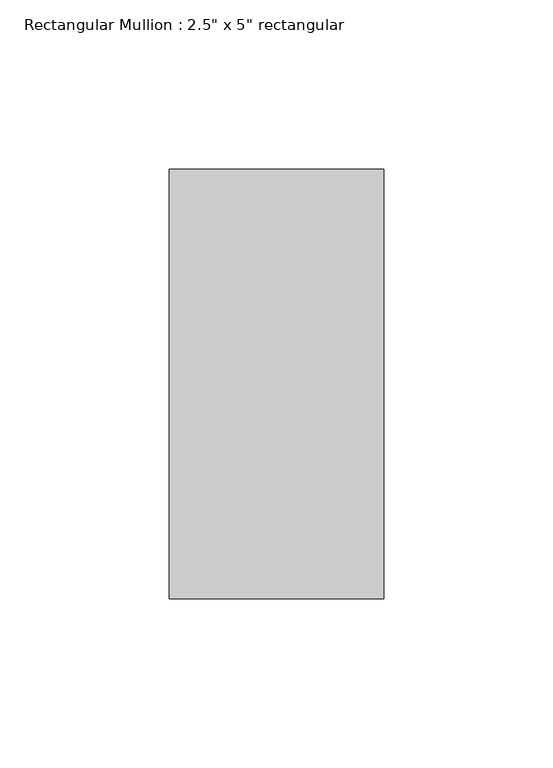
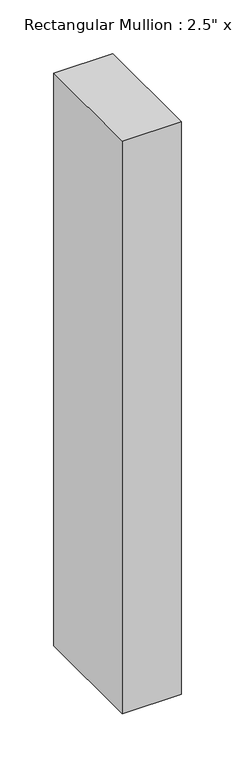
"""IFC4 building model written with IfcOpenShell, lengths in millimetres: member geometry."""

from ifc_helpers import new_model, si_unit, frame, origin, place, context, project, spatial, polyline, outline, extrude, source, transform, mapped, element, save


def member_1d9ef59f(model_context):
    return source(origin(), model_context, "Body", "SweptSolid", [
        extrude(outline(polyline([(0.0, 63.5), (0.0, -63.5), (-63.5, -63.5), (-63.5, 63.5), (0.0, 63.5)])), frame((0.0, 0.0, -650.4541417), z_axis=(0.0, 0.0, 1.0), x_axis=(1.0, 0.0, 0.0)), (0.0, 0.0, 1.0), 650.4541417),
    ])


if __name__ == "__main__":
    model = new_model("IFC4")
    model_context = context("Model", 3, world=origin())
    ifc_project = project(units=[si_unit("LENGTHUNIT", "METRE", prefix="MILLI")], contexts=[model_context])
    site = spatial("IfcSite", under=ifc_project)
    building = spatial("IfcBuilding", under=site)
    placement = place(None, origin())
    member_shape = member_1d9ef59f(model_context)
    element("IfcMember", 1, ObjectType="Rectangular Mullion : 2.5\" x 5\" rectangular", at=placement, inside=building, context=model_context, shape_type="MappedRepresentation", body=[
        mapped(member_shape, transform((0.0, 0.0, 0.0), x_axis=(1.0, 0.0, 0.0), y_axis=(0.0, 1.0, 0.0), z_axis=(0.0, 0.0, 1.0))),
    ])
    save(model, "model.ifc")

# Revit data of these elements
# Type "Rectangular Mullion : 2.5\" x 5\" rectangular"
#   built-in parameter 1007304 = 0.416667 (stored number, unit not read)
#   built-in parameter 1007301 = 0.104167 (stored number, unit not read)
#   built-in parameter 1007300 = 0.104167 (stored number, unit not read)
# Element 1 (IfcMember, "Rectangular Mullion : 2.5\" x 5\" rectangular")
#   Materials on its faces: "Aluminum"
# Materials
#   "Aluminum": class "Metal", colour RGB 247 247 247, transparency 0, Description = "Aluminum 6061", Cost = 0
